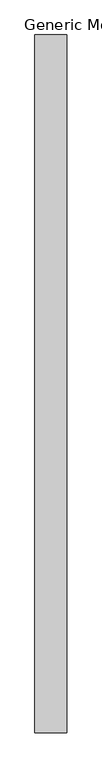
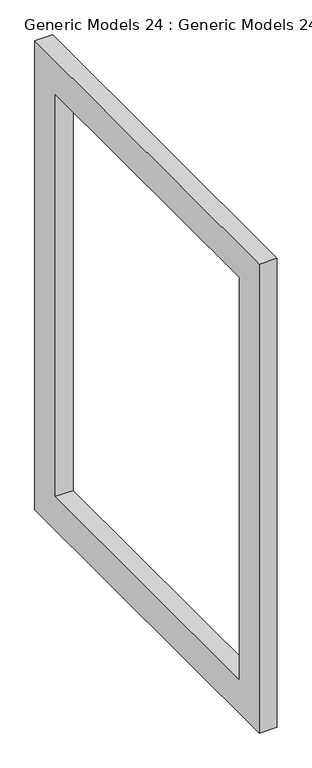
"""IFC4 building model written with IfcOpenShell, lengths in millimetres: proxy geometry, Generic Models 24 : Generic Models 24."""

from ifc_helpers import new_model, si_unit, frame, origin, place, context, project, spatial, polyline, outline, extrude, source, transform, mapped, element, save


def generic_models_24_generic_models_24_8205a677(model_context):
    return source(origin(), model_context, "Body", "SweptSolid", [
        extrude(outline(polyline([(3459.3857468, 8636.0), (4576.9857468, 8636.0), (4576.9857468, 7213.6), (3459.3857468, 7213.6), (3459.3857468, 8636.0)]), holes=[polyline([(3560.9857468, 8534.4), (3560.9857468, 7315.2), (4475.3857468, 7315.2), (4475.3857468, 8534.4), (3560.9857468, 8534.4)])]), frame((-10043.3781265, 0.0, 0.0), z_axis=(1.0, 0.0, 0.0), x_axis=(0.0, 1.0, 0.0)), (0.0, 0.0, 1.0), 50.8),
    ])


if __name__ == "__main__":
    model = new_model("IFC4")
    model_context = context("Model", 3, world=origin())
    ifc_project = project(units=[si_unit("LENGTHUNIT", "METRE", prefix="MILLI")], contexts=[model_context])
    site = spatial("IfcSite", under=ifc_project)
    building = spatial("IfcBuilding", under=site)
    placement = place(None, origin())
    generic_models_24_generic_models_24_shape = generic_models_24_generic_models_24_8205a677(model_context)
    element("IfcBuildingElementProxy", 1, Name="Generic Models 24 : Generic Models 24", ObjectType="Generic Models 24 : Generic Models 24", at=placement, inside=building, context=model_context, shape_type="MappedRepresentation", body=[
        mapped(generic_models_24_generic_models_24_shape, transform((0.0, 0.0, 0.0), x_axis=(1.0, 0.0, 0.0), y_axis=(0.0, 1.0, 0.0), z_axis=(0.0, 0.0, 1.0))),
    ])
    save(model, "model.ifc")
